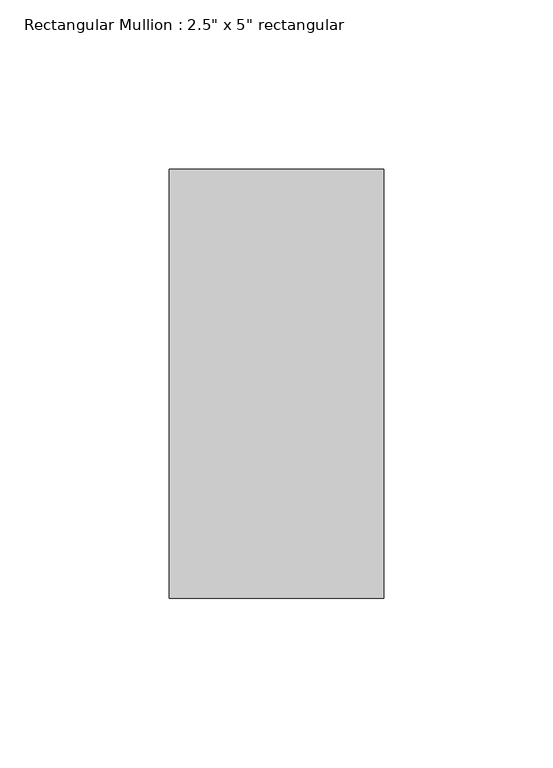
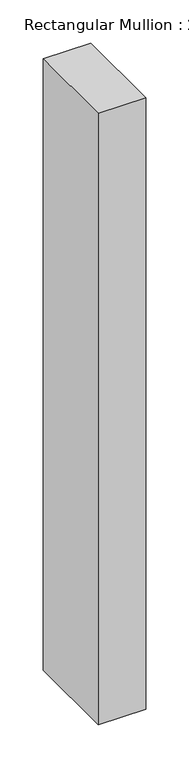
"""IFC4 building model written with IfcOpenShell, lengths in millimetres: member geometry."""

from ifc_helpers import new_model, si_unit, frame, origin, place, context, project, spatial, polyline, outline, extrude, source, transform, mapped, element, save


def member_fd92426f(model_context):
    return source(origin(), model_context, "Body", "SweptSolid", [
        extrude(outline(polyline([(31.75, 63.5), (31.75, -63.5), (-31.75, -63.5), (-31.75, 63.5), (31.75, 63.5)])), frame((0.0, 0.0, -863.6), z_axis=(0.0, 0.0, 1.0), x_axis=(1.0, 0.0, 0.0)), (0.0, 0.0, 1.0), 863.6),
    ])


if __name__ == "__main__":
    model = new_model("IFC4")
    model_context = context("Model", 3, world=origin())
    ifc_project = project(units=[si_unit("LENGTHUNIT", "METRE", prefix="MILLI")], contexts=[model_context])
    site = spatial("IfcSite", under=ifc_project)
    building = spatial("IfcBuilding", under=site)
    placement = place(None, origin())
    member_shape = member_fd92426f(model_context)
    element("IfcMember", 1, ObjectType="Rectangular Mullion : 2.5\" x 5\" rectangular", at=placement, inside=building, context=model_context, shape_type="MappedRepresentation", body=[
        mapped(member_shape, transform((0.0, 0.0, 0.0), x_axis=(1.0, 0.0, 0.0), y_axis=(0.0, 1.0, 0.0), z_axis=(0.0, 0.0, 1.0))),
    ])
    save(model, "model.ifc")

# Revit data of these elements
# Type "Rectangular Mullion : 2.5\" x 5\" rectangular"
#   built-in parameter 1007304 = 0.416667 (stored number, unit not read)
#   built-in parameter 1007301 = 0.104167 (stored number, unit not read)
#   built-in parameter 1007300 = 0.104167 (stored number, unit not read)
# Element 1 (IfcMember, "Rectangular Mullion : 2.5\" x 5\" rectangular")
#   Materials on its faces: "door colour"
# Materials
#   "door colour": class "Generic", colour RGB 120 120 120, transparency 0, Cost = 0
